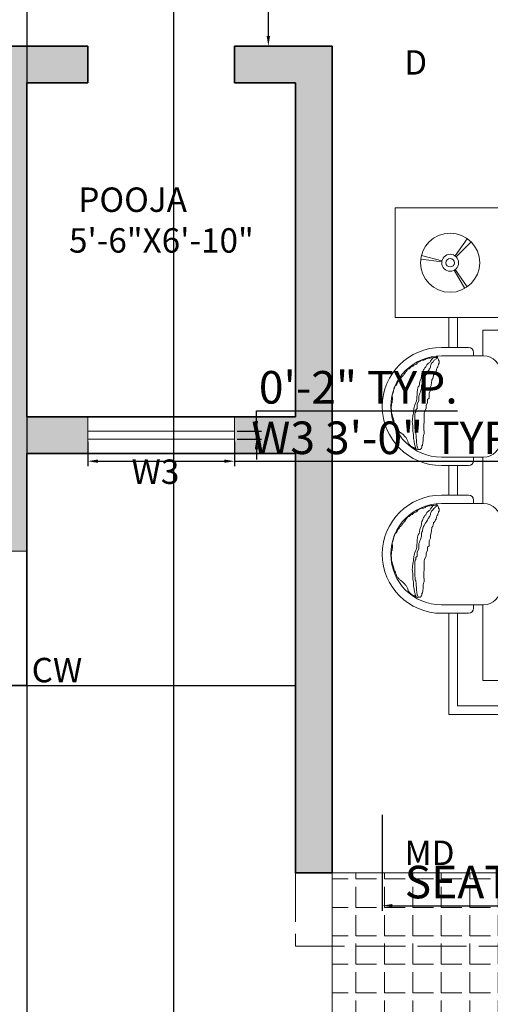
# Model space of a CAD drawing. Units: inches. Extents: x 1070 to 2371, y 645 to 1546.
# Tile 3 of 10: x 1342 to 1458, y 772 to 1014. Entities that reach past the tile are written whole.
import ezdxf

# ---------------------------------------------------------------- set-up
doc = ezdxf.new("R2010")
doc.units = ezdxf.units.IN
doc.linetypes.add('ACAD_ISO02W100', pattern=[15, 12, -3])
for name, color, linetype, lineweight in [('A-ANNO-DIMS', 2, 'Continuous', 18), ('A-ANNO-TEXT', 7, 'Continuous', 18), ('A-AREA-IDEN', 7, 'Continuous', 18), ('A-DOOR', 4, 'Continuous', 18), ('A-FLOR', 7, 'Continuous', 25), ('A-FURN', 8, 'Continuous', 18), ('A-GLAZ', 4, 'Continuous', 18), ('A-ROOF-OVHD', 8, 'ACAD_ISO02W100', 13), ('A-WALL', 7, 'Continuous', 35), ('L-PLNT-BEDS', 3, 'Continuous', 18), ('L-TURF-PATT', 9, 'Continuous', 13)]:
    doc.layers.add(name, color=color, linetype=linetype, lineweight=lineweight)
doc.layers.add('A-WALL-PATT', color=162, linetype='Continuous', lineweight=13, true_color=0x044ac3)
doc.styles.get("Standard").update_dxf_attribs({"font": 'arial.ttf'})
doc.dimstyles.new('ISO-25', dxfattribs={"dimtxt": 8, "dimasz": 2.5, "dimexe": 1.25, "dimexo": 0.625, "dimtad": 1, "dimtih": 1, "dimtoh": 1, "dimdec": 1, "dimlunit": 3, "dimtxsty": 'Standard', "dimcen": 2.5, "dimadec": 0, "dimazin": 0, "dimtfac": 1, "dimtdec": 1, "dimtmove": 0, "dimatfit": 3, "dimfxl": 1, "dimarcsym": 0})

# ---------------------------------------------------------------- blocks, each defined once
blk = doc.blocks.new('A$C71DE5BFE')
for p, q in [((430.7, 3295.7), (503.4, 3397.4)), ((437, 3290.4), (525.4, 3378.7)), ((352, 3261.2), (228, 3276.7)), ((353.2, 3267.1), (231.9, 3297.4)), ((426.5, 3211.6), (488.5, 3103.1)), ((430.7, 3214.3), (503.4, 3112.6)), ((394.4, 2753.9), (394.4, 2930)), ((444.4, 2753.9), (444.4, 2930)), ((350, 2753.9), (510, 2753.9)), ((254.6, 2681.5), (256.9, 2686.1)), ((256.9, 2686.1), (261.2, 2686.1)), ((261.2, 2686.1), (265.5, 2688.1)), ((265.5, 2688.1), (270.1, 2688.1)), ((270.1, 2688.1), (274.4, 2690.5)), ((274.4, 2690.5), (283.1, 2690.5)), ((283.1, 2690.5), (287.7, 2692.5)), ((287.7, 2692.5), (305, 2692.5)), ((292, 2681.5), (296.3, 2686.1)), ((296.3, 2686.1), (298.6, 2690.5)), ((298.6, 2690.5), (300.7, 2694.8)), ((300.7, 2694.8), (303, 2694.8)), ((305, 2692.5), (309.6, 2694.8)), ((309.6, 2694.8), (322.6, 2694.8)), ((315.9, 2683.8), (311.6, 2681.5)), ((320.5, 2686.1), (315.9, 2683.8)), ((318.2, 2697.1), (322.6, 2697.1)), ((322.6, 2690.5), (320.5, 2686.1)), ((322.6, 2694.8), (326.9, 2697.1)), ((322.6, 2697.1), (326.9, 2694.8)), ((326.9, 2694.8), (322.6, 2690.5)), ((326.9, 2697.1), (329.2, 2697.1)), ((326.9, 2694.8), (331.5, 2686.1)), ((331.5, 2686.1), (333.5, 2681.5)), ((350, 2703.9), (600, 2703.9)), ((540, 2723.9), (540, 2703.9)), ((149.4, 2622.4), (154, 2624.7)), ((154, 2624.7), (158.3, 2626.7)), ((158.3, 2626.7), (162.6, 2631.3)), ((162.6, 2631.3), (166.9, 2635.6)), ((166.9, 2635.6), (171.3, 2637.7)), ((171.3, 2637.7), (175.9, 2640)), ((175.9, 2640), (180.2, 2642.3)), ((180.2, 2642.3), (184.5, 2646.6)), ((184.5, 2646.6), (188.8, 2648.6)), ((188.8, 2648.6), (193.5, 2650.9)), ((193.5, 2650.9), (197.8, 2653.2)), ((197.8, 2653.2), (202.1, 2655.3)), ((202.1, 2655.3), (206.4, 2659.6)), ((206.4, 2659.6), (210.7, 2661.9)), ((210.7, 2661.9), (213.1, 2666.2)), ((213.1, 2666.2), (217.4, 2668.5)), ((217.4, 2668.5), (219.7, 2672.9)), ((219.7, 2672.9), (224, 2672.9)), ((224, 2672.9), (228.3, 2675.2)), ((228.3, 2675.2), (232.7, 2677.2)), ((232.7, 2677.2), (245.9, 2677.2)), ((243.6, 2620.4), (248.2, 2624.7)), ((245.9, 2677.2), (250.2, 2679.5)), ((248.2, 2624.7), (250.2, 2629)), ((250.2, 2679.5), (254.6, 2681.5)), ((250.2, 2629), (252.5, 2633.3)), ((252.5, 2633.3), (256.9, 2637.7)), ((256.9, 2637.7), (259.2, 2642.3)), ((259.2, 2642.3), (261.2, 2646.6)), ((261.2, 2646.6), (263.5, 2650.9)), ((263.5, 2650.9), (267.8, 2655.3)), ((267.8, 2655.3), (272.1, 2657.6)), ((272.1, 2657.6), (276.5, 2661.9)), ((276.5, 2661.9), (281.1, 2664.2)), ((281.1, 2629), (276.5, 2624.7)), ((276.5, 2624.7), (276.5, 2620.4)), ((281.1, 2664.2), (283.1, 2668.5)), ((283.1, 2633.3), (281.1, 2629)), ((283.1, 2668.5), (285.4, 2672.9)), ((285.4, 2637.7), (283.1, 2633.3)), ((285.4, 2672.9), (289.7, 2677.2)), ((287.7, 2648.6), (285.4, 2644.3)), ((285.4, 2644.3), (285.4, 2637.7)), ((289.7, 2655.3), (287.7, 2648.6)), ((289.7, 2677.2), (292, 2681.5)), ((292, 2659.6), (289.7, 2655.3)), ((296.3, 2664.2), (292, 2659.6)), ((300.7, 2668.5), (296.3, 2664.2)), ((305, 2675.2), (300.7, 2668.5)), ((309.6, 2677.2), (305, 2675.2)), ((311.6, 2681.5), (309.6, 2677.2)), ((322.6, 2629), (320.5, 2624.7)), ((320.5, 2624.7), (320.5, 2620.4)), ((324.9, 2633.3), (322.6, 2629)), ((329.2, 2637.7), (324.9, 2633.3)), ((331.5, 2646.6), (329.2, 2642.3)), ((329.2, 2642.3), (329.2, 2637.7)), ((333.5, 2650.9), (331.5, 2646.6)), ((333.5, 2681.5), (333.5, 2677.2)), ((333.5, 2677.2), (335.8, 2672.9)), ((335.8, 2659.6), (333.5, 2655.3)), ((333.5, 2655.3), (333.5, 2650.9)), ((335.8, 2672.9), (335.8, 2659.6)), ((103.5, 2563.2), (105.6, 2567.6)), ((105.6, 2567.6), (110.2, 2567.6)), ((110.2, 2572.2), (114.5, 2574.2)), ((110.2, 2567.6), (110.2, 2572.2)), ((114.5, 2574.2), (116.5, 2578.5)), ((116.5, 2578.5), (118.8, 2583.1)), ((118.8, 2583.1), (123.1, 2585.2)), ((123.1, 2589.5), (127.5, 2591.8)), ((123.1, 2585.2), (123.1, 2589.5)), ((127.5, 2591.8), (129.8, 2596.1)), ((129.8, 2596.1), (134.1, 2600.5)), ((134.1, 2600.5), (136.4, 2605.1)), ((136.4, 2605.1), (138.4, 2609.4)), ((138.4, 2609.4), (143, 2611.4)), ((143, 2615.7), (147.3, 2618)), ((143, 2611.4), (143, 2615.7)), ((147.3, 2618), (149.4, 2622.4)), ((228.3, 2565.5), (230.6, 2569.9)), ((230.6, 2574.2), (232.7, 2580.8)), ((230.6, 2569.9), (230.6, 2574.2)), ((232.7, 2589.5), (235, 2594.1)), ((232.7, 2580.8), (232.7, 2589.5)), ((235, 2598.4), (237.3, 2602.8)), ((235, 2594.1), (235, 2598.4)), ((237.3, 2602.8), (239.3, 2607.1)), ((239.3, 2611.4), (241.6, 2615.7)), ((239.3, 2607.1), (239.3, 2611.4)), ((241.6, 2615.7), (243.6, 2620.4)), ((243.6, 2567.6), (241.6, 2561.2)), ((248.2, 2574.2), (243.6, 2567.6)), ((250.2, 2578.5), (248.2, 2574.2)), ((254.6, 2585.2), (250.2, 2578.5)), ((259.2, 2594.1), (254.6, 2585.2)), ((267.8, 2605.1), (259.2, 2594.1)), ((272.1, 2615.7), (267.8, 2605.1)), ((276.5, 2620.4), (272.1, 2615.7)), ((298.6, 2569.9), (294, 2561.2)), ((300.7, 2578.5), (298.6, 2569.9)), ((303, 2585.2), (300.7, 2578.5)), ((311.6, 2598.4), (303, 2589.5)), ((303, 2589.5), (303, 2585.2)), ((315.9, 2607.1), (311.6, 2598.4)), ((318.2, 2611.4), (315.9, 2607.1)), ((320.5, 2620.4), (318.2, 2615.7)), ((318.2, 2615.7), (318.2, 2611.4)), ((68.4, 2510.7), (70.7, 2515.1)), ((68.4, 2502.1), (68.4, 2510.7)), ((70.7, 2515.1), (72.7, 2519.4)), ((72.7, 2519.4), (75, 2523.7)), ((75, 2523.7), (79.3, 2528.3)), ((79.3, 2528.3), (83.7, 2530.4)), ((83.7, 2530.4), (86, 2534.7)), ((86, 2534.7), (88.3, 2539.3)), ((88.3, 2539.3), (90.3, 2543.6)), ((90.3, 2543.6), (92.6, 2547.9)), ((92.6, 2547.9), (94.6, 2552.3)), ((94.6, 2552.3), (99.2, 2556.6)), ((99.2, 2561.2), (103.5, 2563.2)), ((99.2, 2556.6), (99.2, 2561.2)), ((208.7, 2506.4), (210.7, 2510.7)), ((210.7, 2515.1), (213.1, 2519.4)), ((210.7, 2510.7), (210.7, 2515.1)), ((213.1, 2519.4), (217.4, 2526)), ((217.4, 2530.4), (219.7, 2534.7)), ((217.4, 2526), (217.4, 2530.4)), ((219.7, 2541.3), (221.7, 2547.9)), ((219.7, 2534.7), (219.7, 2541.3)), ((221.7, 2552.3), (224, 2556.6)), ((221.7, 2547.9), (221.7, 2552.3)), ((224, 2556.6), (226.3, 2561.2)), ((226.3, 2561.2), (228.3, 2565.5)), ((232.7, 2510.7), (230.6, 2504.1)), ((235, 2534.7), (232.7, 2530.4)), ((232.7, 2530.4), (232.7, 2510.7)), ((237.3, 2541.3), (235, 2534.7)), ((239.3, 2552.3), (237.3, 2545.6)), ((237.3, 2545.6), (237.3, 2541.3)), ((241.6, 2561.2), (239.3, 2556.6)), ((239.3, 2556.6), (239.3, 2552.3)), ((289.7, 2528.3), (285.4, 2519.4)), ((285.4, 2519.4), (285.4, 2499.8)), ((292, 2541.3), (289.7, 2534.7)), ((289.7, 2534.7), (289.7, 2528.3)), ((294, 2556.6), (292, 2547.9)), ((292, 2547.9), (292, 2541.3)), ((294, 2561.2), (294, 2556.6)), ((57.4, 2471.2), (59.7, 2475.5)), ((57.4, 2462.6), (57.4, 2471.2)), ((59.7, 2458.2), (57.4, 2462.6)), ((59.7, 2475.5), (61.8, 2480.2)), ((59.7, 2440.6), (59.7, 2458.2)), ((61.8, 2480.2), (64.1, 2484.5)), ((64.1, 2488.8), (66.4, 2493.1)), ((64.1, 2484.5), (64.1, 2488.8)), ((66.4, 2497.5), (68.4, 2502.1)), ((66.4, 2493.1), (66.4, 2497.5)), ((204.4, 2464.6), (206.4, 2469.2)), ((204.4, 2445), (204.4, 2464.6)), ((206.4, 2493.1), (208.7, 2497.5)), ((206.4, 2469.2), (206.4, 2493.1)), ((208.7, 2497.5), (208.7, 2506.4)), ((217.4, 2471.2), (215.4, 2466.9)), ((215.4, 2466.9), (215.4, 2436.3)), ((219.7, 2475.5), (217.4, 2471.2)), ((221.7, 2482.2), (219.7, 2475.5)), ((224, 2486.5), (221.7, 2482.2)), ((226.3, 2491.1), (224, 2486.5)), ((228.3, 2497.5), (226.3, 2491.1)), ((230.6, 2504.1), (228.3, 2497.5)), ((276.5, 2453.6), (267.8, 2445)), ((285.4, 2499.8), (276.5, 2482.2)), ((276.5, 2482.2), (276.5, 2453.6)), ((53.1, 2401.1), (55.1, 2405.4)), ((53.1, 2392.5), (53.1, 2401.1)), ((55.1, 2388.1), (53.1, 2392.5)), ((55.1, 2423), (57.4, 2427.4)), ((55.1, 2405.4), (55.1, 2423)), ((57.4, 2436.3), (59.7, 2440.6)), ((57.4, 2427.4), (57.4, 2436.3)), ((186.8, 2392.5), (188.8, 2396.8)), ((186.8, 2381.5), (186.8, 2392.5)), ((188.8, 2401.1), (191.2, 2405.4)), ((188.8, 2396.8), (188.8, 2401.1)), ((191.2, 2405.4), (193.5, 2414.4)), ((193.5, 2414.4), (197.8, 2427.4)), ((197.8, 2427.4), (199.8, 2431.7)), ((206.4, 2392.5), (197.8, 2383.5)), ((199.8, 2431.7), (202.1, 2436.3)), ((202.1, 2440.6), (204.4, 2445)), ((202.1, 2436.3), (202.1, 2440.6)), ((215.4, 2436.3), (206.4, 2418.7)), ((206.4, 2418.7), (206.4, 2392.5)), ((259.2, 2392.5), (250.2, 2374.9)), ((267.8, 2427.4), (259.2, 2410.1)), ((259.2, 2410.1), (259.2, 2392.5)), ((267.8, 2445), (267.8, 2427.4)), ((55.1, 2361.6), (55.1, 2388.1)), ((57.4, 2357.3), (55.1, 2361.6)), ((57.4, 2352.9), (57.4, 2357.3)), ((59.7, 2348.6), (57.4, 2352.9)), ((59.7, 2344.3), (59.7, 2348.6)), ((61.8, 2340), (59.7, 2344.3)), ((64.1, 2335.3), (61.8, 2340)), ((66.4, 2331), (64.1, 2335.3)), ((177.9, 2335.3), (180.2, 2342)), ((177.9, 2322.4), (177.9, 2335.3)), ((180.2, 2350.6), (182.5, 2357.3)), ((180.2, 2342), (180.2, 2350.6)), ((182.5, 2357.3), (184.5, 2363.9)), ((184.5, 2377.2), (186.8, 2381.5)), ((184.5, 2363.9), (184.5, 2377.2)), ((195.5, 2363.9), (193.5, 2359.6)), ((193.5, 2359.6), (193.5, 2274.2)), ((197.8, 2372.6), (195.5, 2368.2)), ((195.5, 2368.2), (195.5, 2363.9)), ((197.8, 2383.5), (197.8, 2372.6)), ((250.2, 2370.5), (248.2, 2366.2)), ((248.2, 2366.2), (248.2, 2307.1)), ((250.2, 2374.9), (250.2, 2370.5)), ((66.4, 2326.7), (66.4, 2331)), ((68.4, 2322.4), (66.4, 2326.7)), ((68.4, 2318), (68.4, 2322.4)), ((70.7, 2311.4), (68.4, 2318)), ((72.7, 2307.1), (70.7, 2311.4)), ((75, 2302.5), (72.7, 2307.1)), ((77.3, 2298.1), (75, 2302.5)), ((77.3, 2293.8), (77.3, 2298.1)), ((79.3, 2289.5), (77.3, 2293.8)), ((81.6, 2285.1), (79.3, 2289.5)), ((83.7, 2278.5), (81.6, 2285.1)), ((86, 2274.2), (83.7, 2278.5)), ((175.9, 2315.7), (177.9, 2322.4)), ((175.9, 2311.4), (175.9, 2315.7)), ((177.9, 2307.1), (175.9, 2311.4)), ((177.9, 2298.1), (177.9, 2307.1)), ((180.2, 2293.8), (177.9, 2298.1)), ((180.2, 2254.3), (180.2, 2293.8)), ((248.2, 2307.1), (245.9, 2300.4)), ((245.9, 2300.4), (245.9, 2263.2)), ((88.3, 2269.6), (86, 2274.2)), ((90.3, 2265.2), (88.3, 2269.6)), ((94.6, 2263.2), (90.3, 2265.2)), ((96.9, 2258.6), (94.6, 2263.2)), ((101.2, 2256.6), (96.9, 2258.6)), ((103.5, 2252.3), (101.2, 2256.6)), ((107.9, 2250), (103.5, 2252.3)), ((112.2, 2245.6), (107.9, 2250)), ((121.1, 2239), (112.2, 2245.6)), ((134.1, 2226), (121.1, 2239)), ((136.4, 2221.4), (134.1, 2226)), ((140.7, 2219.4), (136.4, 2221.4)), ((143, 2215), (140.7, 2219.4)), ((182.5, 2250), (180.2, 2254.3)), ((182.5, 2245.6), (182.5, 2250)), ((184.5, 2239), (182.5, 2245.6)), ((184.5, 2212.7), (184.5, 2239)), ((193.5, 2274.2), (195.5, 2265.2)), ((195.5, 2265.2), (195.5, 2252.3)), ((195.5, 2252.3), (197.8, 2247.9)), ((197.8, 2247.9), (197.8, 2243.3)), ((197.8, 2243.3), (199.8, 2232.4)), ((199.8, 2232.4), (199.8, 2215)), ((243.6, 2228), (241.6, 2223.7)), ((241.6, 2223.7), (241.6, 2197.5)), ((245.9, 2237), (243.6, 2232.4)), ((243.6, 2232.4), (243.6, 2228)), ((245.9, 2263.2), (248.2, 2258.6)), ((248.2, 2241.3), (245.9, 2237)), ((248.2, 2258.6), (248.2, 2241.3)), ((145, 2210.4), (143, 2215)), ((147.3, 2206.1), (145, 2210.4)), ((149.4, 2201.8), (147.3, 2206.1)), ((151.7, 2197.5), (149.4, 2201.8)), ((154, 2190.8), (151.7, 2197.5)), ((154, 2186.5), (154, 2190.8)), ((156, 2182.2), (154, 2186.5)), ((160.3, 2179.9), (156, 2182.2)), ((162.6, 2175.5), (160.3, 2179.9)), ((166.9, 2171.2), (162.6, 2175.5)), ((169.2, 2166.6), (166.9, 2171.2)), ((173.6, 2166.6), (169.2, 2166.6)), ((175.9, 2162.3), (173.6, 2166.6)), ((180.2, 2162.3), (175.9, 2162.3)), ((184.5, 2160.2), (180.2, 2162.3)), ((186.8, 2208.4), (184.5, 2212.7)), ((188.8, 2157.9), (184.5, 2160.2)), ((186.8, 2204.1), (186.8, 2208.4)), ((188.8, 2199.5), (186.8, 2204.1)), ((188.8, 2190.8), (188.8, 2199.5)), ((191.2, 2186.5), (188.8, 2190.8)), ((195.5, 2153.6), (188.8, 2157.9)), ((191.2, 2179.9), (191.2, 2186.5)), ((193.5, 2175.5), (191.2, 2179.9)), ((195.5, 2171.2), (193.5, 2175.5)), ((195.5, 2162.3), (195.5, 2171.2)), ((197.8, 2157.9), (195.5, 2162.3)), ((199.8, 2153.6), (197.8, 2157.9)), ((199.8, 2215), (202.1, 2208.4)), ((202.1, 2208.4), (202.1, 2186.5)), ((202.1, 2186.5), (204.4, 2182.2)), ((204.4, 2182.2), (204.4, 2173.2)), ((204.4, 2173.2), (206.4, 2168.9)), ((206.4, 2168.9), (206.4, 2164.6)), ((206.4, 2164.6), (208.7, 2160.2)), ((208.7, 2160.2), (210.7, 2155.9)), ((232.7, 2157.9), (228.3, 2153.6)), ((235, 2162.3), (232.7, 2157.9)), ((237.3, 2175.5), (235, 2171.2)), ((235, 2171.2), (235, 2162.3)), ((239.3, 2184.2), (237.3, 2179.9)), ((237.3, 2179.9), (237.3, 2175.5)), ((241.6, 2197.5), (239.3, 2193.1)), ((239.3, 2193.1), (239.3, 2184.2)), ((199.8, 2151.3), (195.5, 2153.6)), ((199.8, 2149.3), (199.8, 2153.6)), ((204.4, 2149.3), (199.8, 2151.3)), ((208.7, 2147), (204.4, 2149.3)), ((213.1, 2149.3), (208.7, 2147)), ((210.7, 2155.9), (213.1, 2151.3)), ((213.1, 2151.3), (213.1, 2149.3)), ((226.3, 2149.3), (213.1, 2149.3)), ((228.3, 2153.6), (226.3, 2149.3)), ((350, 2103.9), (600, 2103.9)), ((540, 2103.9), (540, 2083.9)), ((594.4, 1828.9), (594.4, 2103.9)), ((510, 2053.9), (350, 2053.9)), ((394.4, 1878.9), (394.4, 2053.9)), ((444.4, 1878.9), (444.4, 2053.9)), ((350, 1878.9), (510, 1878.9)), ((254.6, 1806.5), (256.9, 1811.1)), ((256.9, 1811.1), (261.2, 1811.1)), ((261.2, 1811.1), (265.5, 1813.1)), ((265.5, 1813.1), (270.1, 1813.1)), ((270.1, 1813.1), (274.4, 1815.5)), ((274.4, 1815.5), (283.1, 1815.5)), ((283.1, 1815.5), (287.7, 1817.5)), ((287.7, 1817.5), (305, 1817.5)), ((292, 1806.5), (296.3, 1811.1)), ((296.3, 1811.1), (298.6, 1815.5)), ((298.6, 1815.5), (300.7, 1819.8)), ((300.7, 1819.8), (303, 1819.8)), ((305, 1817.5), (309.6, 1819.8)), ((309.6, 1819.8), (322.6, 1819.8)), ((315.9, 1808.8), (311.6, 1806.5)), ((320.5, 1811.1), (315.9, 1808.8)), ((318.2, 1822.1), (322.6, 1822.1)), ((322.6, 1815.5), (320.5, 1811.1)), ((322.6, 1819.8), (326.9, 1822.1)), ((322.6, 1822.1), (326.9, 1819.8)), ((326.9, 1819.8), (322.6, 1815.5)), ((326.9, 1822.1), (329.2, 1822.1)), ((326.9, 1819.8), (331.5, 1811.1)), ((331.5, 1811.1), (333.5, 1806.5)), ((350, 1828.9), (600, 1828.9)), ((540, 1848.9), (540, 1828.9)), ((149.4, 1747.4), (154, 1749.7)), ((154, 1749.7), (158.3, 1751.7)), ((158.3, 1751.7), (162.6, 1756.3)), ((162.6, 1756.3), (166.9, 1760.6)), ((166.9, 1760.6), (171.3, 1762.7)), ((171.3, 1762.7), (175.9, 1765)), ((175.9, 1765), (180.2, 1767.3)), ((180.2, 1767.3), (184.5, 1771.6)), ((184.5, 1771.6), (188.8, 1773.6)), ((188.8, 1773.6), (193.5, 1775.9)), ((193.5, 1775.9), (197.8, 1778.2)), ((197.8, 1778.2), (202.1, 1780.3)), ((202.1, 1780.3), (206.4, 1784.6)), ((206.4, 1784.6), (210.7, 1786.9)), ((210.7, 1786.9), (213.1, 1791.2)), ((213.1, 1791.2), (217.4, 1793.5)), ((217.4, 1793.5), (219.7, 1797.9)), ((219.7, 1797.9), (224, 1797.9)), ((224, 1797.9), (228.3, 1800.2)), ((228.3, 1800.2), (232.7, 1802.2)), ((232.7, 1802.2), (245.9, 1802.2)), ((243.6, 1745.4), (248.2, 1749.7)), ((245.9, 1802.2), (250.2, 1804.5)), ((248.2, 1749.7), (250.2, 1754)), ((250.2, 1804.5), (254.6, 1806.5)), ((250.2, 1754), (252.5, 1758.3)), ((252.5, 1758.3), (256.9, 1762.7)), ((256.9, 1762.7), (259.2, 1767.3)), ((259.2, 1767.3), (261.2, 1771.6)), ((261.2, 1771.6), (263.5, 1775.9)), ((263.5, 1775.9), (267.8, 1780.3)), ((267.8, 1780.3), (272.1, 1782.6)), ((272.1, 1782.6), (276.5, 1786.9)), ((276.5, 1786.9), (281.1, 1789.2)), ((281.1, 1754), (276.5, 1749.7)), ((276.5, 1749.7), (276.5, 1745.4)), ((281.1, 1789.2), (283.1, 1793.5)), ((283.1, 1758.3), (281.1, 1754)), ((283.1, 1793.5), (285.4, 1797.9)), ((285.4, 1762.7), (283.1, 1758.3)), ((285.4, 1797.9), (289.7, 1802.2)), ((287.7, 1773.6), (285.4, 1769.3)), ((285.4, 1769.3), (285.4, 1762.7)), ((289.7, 1780.3), (287.7, 1773.6)), ((289.7, 1802.2), (292, 1806.5)), ((292, 1784.6), (289.7, 1780.3)), ((296.3, 1789.2), (292, 1784.6)), ((300.7, 1793.5), (296.3, 1789.2)), ((305, 1800.2), (300.7, 1793.5)), ((309.6, 1802.2), (305, 1800.2)), ((311.6, 1806.5), (309.6, 1802.2)), ((322.6, 1754), (320.5, 1749.7)), ((320.5, 1749.7), (320.5, 1745.4)), ((324.9, 1758.3), (322.6, 1754)), ((329.2, 1762.7), (324.9, 1758.3)), ((331.5, 1771.6), (329.2, 1767.3)), ((329.2, 1767.3), (329.2, 1762.7)), ((333.5, 1775.9), (331.5, 1771.6)), ((333.5, 1806.5), (333.5, 1802.2)), ((333.5, 1802.2), (335.8, 1797.9)), ((335.8, 1784.6), (333.5, 1780.3)), ((333.5, 1780.3), (333.5, 1775.9)), ((335.8, 1797.9), (335.8, 1784.6)), ((103.5, 1688.2), (105.6, 1692.6)), ((105.6, 1692.6), (110.2, 1692.6)), ((110.2, 1697.2), (114.5, 1699.2)), ((110.2, 1692.6), (110.2, 1697.2)), ((114.5, 1699.2), (116.5, 1703.5)), ((116.5, 1703.5), (118.8, 1708.1)), ((118.8, 1708.1), (123.1, 1710.2)), ((123.1, 1714.5), (127.5, 1716.8)), ((123.1, 1710.2), (123.1, 1714.5)), ((127.5, 1716.8), (129.8, 1721.1)), ((129.8, 1721.1), (134.1, 1725.5)), ((134.1, 1725.5), (136.4, 1730.1)), ((136.4, 1730.1), (138.4, 1734.4)), ((138.4, 1734.4), (143, 1736.4)), ((143, 1740.7), (147.3, 1743)), ((143, 1736.4), (143, 1740.7)), ((147.3, 1743), (149.4, 1747.4)), ((228.3, 1690.5), (230.6, 1694.9)), ((230.6, 1699.2), (232.7, 1705.8)), ((230.6, 1694.9), (230.6, 1699.2)), ((232.7, 1714.5), (235, 1719.1)), ((232.7, 1705.8), (232.7, 1714.5)), ((235, 1723.4), (237.3, 1727.8)), ((235, 1719.1), (235, 1723.4)), ((237.3, 1727.8), (239.3, 1732.1)), ((239.3, 1736.4), (241.6, 1740.7)), ((239.3, 1732.1), (239.3, 1736.4)), ((241.6, 1740.7), (243.6, 1745.4)), ((243.6, 1692.6), (241.6, 1686.2)), ((248.2, 1699.2), (243.6, 1692.6)), ((250.2, 1703.5), (248.2, 1699.2)), ((254.6, 1710.2), (250.2, 1703.5)), ((259.2, 1719.1), (254.6, 1710.2)), ((267.8, 1730.1), (259.2, 1719.1)), ((272.1, 1740.7), (267.8, 1730.1)), ((276.5, 1745.4), (272.1, 1740.7)), ((298.6, 1694.9), (294, 1686.2)), ((300.7, 1703.5), (298.6, 1694.9)), ((303, 1710.2), (300.7, 1703.5)), ((311.6, 1723.4), (303, 1714.5)), ((303, 1714.5), (303, 1710.2)), ((315.9, 1732.1), (311.6, 1723.4)), ((318.2, 1736.4), (315.9, 1732.1)), ((320.5, 1745.4), (318.2, 1740.7)), ((318.2, 1740.7), (318.2, 1736.4)), ((68.4, 1635.7), (70.7, 1640.1)), ((68.4, 1627.1), (68.4, 1635.7)), ((70.7, 1640.1), (72.7, 1644.4)), ((72.7, 1644.4), (75, 1648.7)), ((75, 1648.7), (79.3, 1653.3)), ((79.3, 1653.3), (83.7, 1655.4)), ((83.7, 1655.4), (86, 1659.7)), ((86, 1659.7), (88.3, 1664.3)), ((88.3, 1664.3), (90.3, 1668.6)), ((90.3, 1668.6), (92.6, 1672.9)), ((92.6, 1672.9), (94.6, 1677.3)), ((94.6, 1677.3), (99.2, 1681.6)), ((99.2, 1686.2), (103.5, 1688.2)), ((99.2, 1681.6), (99.2, 1686.2)), ((208.7, 1631.4), (210.7, 1635.7)), ((210.7, 1640.1), (213.1, 1644.4)), ((210.7, 1635.7), (210.7, 1640.1)), ((213.1, 1644.4), (217.4, 1651)), ((217.4, 1655.4), (219.7, 1659.7)), ((217.4, 1651), (217.4, 1655.4)), ((219.7, 1666.3), (221.7, 1672.9)), ((219.7, 1659.7), (219.7, 1666.3)), ((221.7, 1677.3), (224, 1681.6)), ((221.7, 1672.9), (221.7, 1677.3)), ((224, 1681.6), (226.3, 1686.2)), ((226.3, 1686.2), (228.3, 1690.5)), ((232.7, 1635.7), (230.6, 1629.1)), ((235, 1659.7), (232.7, 1655.4)), ((232.7, 1655.4), (232.7, 1635.7)), ((237.3, 1666.3), (235, 1659.7)), ((239.3, 1677.3), (237.3, 1670.6)), ((237.3, 1670.6), (237.3, 1666.3)), ((241.6, 1686.2), (239.3, 1681.6)), ((239.3, 1681.6), (239.3, 1677.3)), ((289.7, 1653.3), (285.4, 1644.4)), ((285.4, 1644.4), (285.4, 1624.8)), ((292, 1666.3), (289.7, 1659.7)), ((289.7, 1659.7), (289.7, 1653.3)), ((294, 1681.6), (292, 1672.9)), ((292, 1672.9), (292, 1666.3)), ((294, 1686.2), (294, 1681.6)), ((57.4, 1596.2), (59.7, 1600.5)), ((57.4, 1587.6), (57.4, 1596.2)), ((59.7, 1583.2), (57.4, 1587.6)), ((59.7, 1600.5), (61.8, 1605.2)), ((59.7, 1565.6), (59.7, 1583.2)), ((61.8, 1605.2), (64.1, 1609.5)), ((64.1, 1613.8), (66.4, 1618.1)), ((64.1, 1609.5), (64.1, 1613.8)), ((66.4, 1622.5), (68.4, 1627.1)), ((66.4, 1618.1), (66.4, 1622.5)), ((204.4, 1589.6), (206.4, 1594.2)), ((204.4, 1570), (204.4, 1589.6)), ((206.4, 1618.1), (208.7, 1622.5)), ((206.4, 1594.2), (206.4, 1618.1)), ((208.7, 1622.5), (208.7, 1631.4)), ((217.4, 1596.2), (215.4, 1591.9)), ((215.4, 1591.9), (215.4, 1561.3)), ((219.7, 1600.5), (217.4, 1596.2)), ((221.7, 1607.2), (219.7, 1600.5)), ((224, 1611.5), (221.7, 1607.2)), ((226.3, 1616.1), (224, 1611.5)), ((228.3, 1622.5), (226.3, 1616.1)), ((230.6, 1629.1), (228.3, 1622.5)), ((276.5, 1578.6), (267.8, 1570)), ((285.4, 1624.8), (276.5, 1607.2)), ((276.5, 1607.2), (276.5, 1578.6)), ((53.1, 1526.1), (55.1, 1530.4)), ((53.1, 1517.5), (53.1, 1526.1)), ((55.1, 1513.1), (53.1, 1517.5)), ((55.1, 1548), (57.4, 1552.4)), ((55.1, 1530.4), (55.1, 1548)), ((57.4, 1561.3), (59.7, 1565.6)), ((57.4, 1552.4), (57.4, 1561.3)), ((186.8, 1517.5), (188.8, 1521.8)), ((186.8, 1506.5), (186.8, 1517.5)), ((188.8, 1526.1), (191.2, 1530.4)), ((188.8, 1521.8), (188.8, 1526.1)), ((191.2, 1530.4), (193.5, 1539.4)), ((193.5, 1539.4), (197.8, 1552.4)), ((197.8, 1552.4), (199.8, 1556.7)), ((206.4, 1517.5), (197.8, 1508.5)), ((199.8, 1556.7), (202.1, 1561.3)), ((202.1, 1565.6), (204.4, 1570)), ((202.1, 1561.3), (202.1, 1565.6)), ((215.4, 1561.3), (206.4, 1543.7)), ((206.4, 1543.7), (206.4, 1517.5)), ((259.2, 1517.5), (250.2, 1499.9)), ((267.8, 1552.4), (259.2, 1535.1)), ((259.2, 1535.1), (259.2, 1517.5)), ((267.8, 1570), (267.8, 1552.4)), ((55.1, 1486.6), (55.1, 1513.1)), ((57.4, 1482.3), (55.1, 1486.6)), ((57.4, 1477.9), (57.4, 1482.3)), ((59.7, 1473.6), (57.4, 1477.9)), ((59.7, 1469.3), (59.7, 1473.6)), ((61.8, 1465), (59.7, 1469.3)), ((64.1, 1460.3), (61.8, 1465)), ((66.4, 1456), (64.1, 1460.3)), ((177.9, 1460.3), (180.2, 1467)), ((177.9, 1447.4), (177.9, 1460.3)), ((180.2, 1475.6), (182.5, 1482.3)), ((180.2, 1467), (180.2, 1475.6)), ((182.5, 1482.3), (184.5, 1488.9)), ((184.5, 1502.2), (186.8, 1506.5)), ((184.5, 1488.9), (184.5, 1502.2)), ((195.5, 1488.9), (193.5, 1484.6)), ((193.5, 1484.6), (193.5, 1399.2)), ((197.8, 1497.6), (195.5, 1493.2)), ((195.5, 1493.2), (195.5, 1488.9)), ((197.8, 1508.5), (197.8, 1497.6)), ((250.2, 1495.5), (248.2, 1491.2)), ((248.2, 1491.2), (248.2, 1432.1)), ((250.2, 1499.9), (250.2, 1495.5)), ((66.4, 1451.7), (66.4, 1456)), ((68.4, 1447.4), (66.4, 1451.7)), ((68.4, 1443), (68.4, 1447.4)), ((70.7, 1436.4), (68.4, 1443)), ((72.7, 1432.1), (70.7, 1436.4)), ((75, 1427.5), (72.7, 1432.1)), ((77.3, 1423.1), (75, 1427.5)), ((77.3, 1418.8), (77.3, 1423.1)), ((79.3, 1414.5), (77.3, 1418.8)), ((81.6, 1410.1), (79.3, 1414.5)), ((83.7, 1403.5), (81.6, 1410.1)), ((86, 1399.2), (83.7, 1403.5)), ((175.9, 1440.7), (177.9, 1447.4)), ((175.9, 1436.4), (175.9, 1440.7)), ((177.9, 1432.1), (175.9, 1436.4)), ((177.9, 1423.1), (177.9, 1432.1)), ((180.2, 1418.8), (177.9, 1423.1)), ((180.2, 1379.3), (180.2, 1418.8)), ((248.2, 1432.1), (245.9, 1425.4)), ((245.9, 1425.4), (245.9, 1388.2)), ((88.3, 1394.6), (86, 1399.2)), ((90.3, 1390.2), (88.3, 1394.6)), ((94.6, 1388.2), (90.3, 1390.2)), ((96.9, 1383.6), (94.6, 1388.2)), ((101.2, 1381.6), (96.9, 1383.6)), ((103.5, 1377.3), (101.2, 1381.6)), ((107.9, 1375), (103.5, 1377.3)), ((112.2, 1370.6), (107.9, 1375)), ((121.1, 1364), (112.2, 1370.6)), ((134.1, 1351), (121.1, 1364)), ((136.4, 1346.4), (134.1, 1351)), ((140.7, 1344.4), (136.4, 1346.4)), ((143, 1340), (140.7, 1344.4)), ((182.5, 1375), (180.2, 1379.3)), ((182.5, 1370.6), (182.5, 1375)), ((184.5, 1364), (182.5, 1370.6)), ((184.5, 1337.7), (184.5, 1364)), ((193.5, 1399.2), (195.5, 1390.2)), ((195.5, 1390.2), (195.5, 1377.3)), ((195.5, 1377.3), (197.8, 1372.9)), ((197.8, 1372.9), (197.8, 1368.3)), ((197.8, 1368.3), (199.8, 1357.4)), ((199.8, 1357.4), (199.8, 1340)), ((243.6, 1353), (241.6, 1348.7)), ((241.6, 1348.7), (241.6, 1322.5)), ((245.9, 1362), (243.6, 1357.4)), ((243.6, 1357.4), (243.6, 1353)), ((245.9, 1388.2), (248.2, 1383.6)), ((248.2, 1366.3), (245.9, 1362)), ((248.2, 1383.6), (248.2, 1366.3)), ((145, 1335.4), (143, 1340)), ((147.3, 1331.1), (145, 1335.4)), ((149.4, 1326.8), (147.3, 1331.1)), ((151.7, 1322.5), (149.4, 1326.8)), ((154, 1315.8), (151.7, 1322.5)), ((154, 1311.5), (154, 1315.8)), ((156, 1307.2), (154, 1311.5)), ((160.3, 1304.9), (156, 1307.2)), ((162.6, 1300.5), (160.3, 1304.9)), ((166.9, 1296.2), (162.6, 1300.5)), ((169.2, 1291.6), (166.9, 1296.2)), ((173.6, 1291.6), (169.2, 1291.6)), ((175.9, 1287.3), (173.6, 1291.6)), ((180.2, 1287.3), (175.9, 1287.3)), ((184.5, 1285.2), (180.2, 1287.3)), ((186.8, 1333.4), (184.5, 1337.7)), ((188.8, 1282.9), (184.5, 1285.2)), ((186.8, 1329.1), (186.8, 1333.4)), ((188.8, 1324.5), (186.8, 1329.1)), ((188.8, 1315.8), (188.8, 1324.5)), ((191.2, 1311.5), (188.8, 1315.8)), ((195.5, 1278.6), (188.8, 1282.9)), ((191.2, 1304.9), (191.2, 1311.5)), ((193.5, 1300.5), (191.2, 1304.9)), ((195.5, 1296.2), (193.5, 1300.5)), ((195.5, 1287.3), (195.5, 1296.2)), ((197.8, 1282.9), (195.5, 1287.3)), ((199.8, 1278.6), (197.8, 1282.9)), ((199.8, 1340), (202.1, 1333.4)), ((202.1, 1333.4), (202.1, 1311.5)), ((202.1, 1311.5), (204.4, 1307.2)), ((204.4, 1307.2), (204.4, 1298.2)), ((204.4, 1298.2), (206.4, 1293.9)), ((206.4, 1293.9), (206.4, 1289.6)), ((206.4, 1289.6), (208.7, 1285.2)), ((208.7, 1285.2), (210.7, 1280.9)), ((232.7, 1282.9), (228.3, 1278.6)), ((235, 1287.3), (232.7, 1282.9)), ((237.3, 1300.5), (235, 1296.2)), ((235, 1296.2), (235, 1287.3)), ((239.3, 1309.2), (237.3, 1304.9)), ((237.3, 1304.9), (237.3, 1300.5)), ((241.6, 1322.5), (239.3, 1318.1)), ((239.3, 1318.1), (239.3, 1309.2)), ((199.8, 1276.3), (195.5, 1278.6)), ((199.8, 1274.3), (199.8, 1278.6)), ((204.4, 1274.3), (199.8, 1276.3)), ((208.7, 1272), (204.4, 1274.3)), ((213.1, 1274.3), (208.7, 1272)), ((210.7, 1280.9), (213.1, 1276.3)), ((213.1, 1276.3), (213.1, 1274.3)), ((226.3, 1274.3), (213.1, 1274.3)), ((228.3, 1278.6), (226.3, 1274.3)), ((350, 1228.9), (600, 1228.9)), ((540, 1228.9), (540, 1208.9)), ((510, 1178.9), (350, 1178.9))]:
    blk.add_line(p, q)
blk.add_lwpolyline([(726.7, 2930), (76.7, 2930), (76.7, 3580), (726.7, 3580)], close=True)
for points in [[(594.4, 2703.9), (594.4, 2855), (953, 2855)], [(1142.3, 780), (594.4, 780), (594.4, 1228.9)], [(1142.3, 580), (394.4, 580), (394.4, 1178.9)], [(1142.3, 630), (444.4, 630), (444.4, 1178.9)]]:
    blk.add_lwpolyline(points)
for radius in [175, 50, 25]:
    blk.add_circle((401.7, 3255), radius)
for centre, radius, start, end in [((350, 2403.9), 350, 90, 270), ((510, 2723.9), 30, 0, 90), ((350, 2403.9), 300, 90.00002, 269.99998), ((600, 2603.9), 100, 0, 90), ((600, 2203.9), 100, 270, 0), ((510, 2083.9), 30, 270, 0), ((350, 1528.9), 350, 90, 270), ((510, 1848.9), 30, 0, 90), ((350, 1528.9), 300, 90.00002, 269.99998), ((600, 1728.9), 100, 0, 90), ((600, 1328.9), 100, 270, 0), ((510, 1208.9), 30, 270, 0)]:
    blk.add_arc(centre, radius, start, end)
blk = doc.blocks.new('*D14')
at = {"layer": 'A-ANNO-DIMS', "color": 0, "lineweight": -2, "transparency": 16777216}
for p, q in [((1383.51, 1049.77), (1404.69, 1049.77)), ((1403.44, 1047.27), (1403.44, 1033.48)), ((1403.44, 1010.27), (1403.44, 1024.06)), ((1395.74, 1007.77), (1404.69, 1007.77))]:
    blk.add_line(p, q, dxfattribs=at)
at = {"layer": 'A-ANNO-DIMS', "color": 0, "transparency": 16777216}
for points in [[(1403.02, 1047.27), (1403.86, 1047.27), (1403.44, 1049.77)], [(1403.02, 1010.27), (1403.86, 1010.27), (1403.44, 1007.77)]]:
    blk.add_solid(points, dxfattribs=at)
at = {"layer": 'Defpoints', "color": 0, "transparency": 16777216}
for p in [(1382.88, 1049.77), (1395.11, 1007.77), (1403.44, 1007.77)]:
    blk.add_point(p, dxfattribs=at)
at = {"layer": 'A-ANNO-DIMS', "color": 0, "transparency": 16777216, "insert": (1403.44, 1028.77), "char_height": 8, "attachment_point": 5}
blk.add_mtext('3\'-6"', dxfattribs=at)
blk = doc.blocks.new('GLAZ-36IN')
for p, q in [((0, 2), (36, 2)), ((0, 0), (36, 0))]:
    blk.add_line(p, q)
blk = doc.blocks.new('*D35')
at = {"layer": 'A-ANNO-DIMS', "color": 0, "lineweight": -2, "transparency": 16777216}
for p, q in [((1431.43, 819.01), (1431.43, 795.46)), ((1584.23, 819.01), (1584.23, 795.46)), ((1433.93, 796.71), (1581.73, 796.71))]:
    blk.add_line(p, q, dxfattribs=at)
at = {"layer": 'A-ANNO-DIMS', "color": 0, "transparency": 16777216}
for points in [[(1433.93, 797.13), (1433.93, 796.3), (1431.43, 796.71)], [(1581.73, 797.13), (1581.73, 796.3), (1584.23, 796.71)]]:
    blk.add_solid(points, dxfattribs=at)
at = {"layer": 'Defpoints', "color": 0, "transparency": 16777216}
for p in [(1431.43, 819.63), (1584.23, 819.63), (1584.23, 796.71)]:
    blk.add_point(p, dxfattribs=at)
at = {"layer": 'A-ANNO-DIMS', "color": 0, "transparency": 16777216, "insert": (1507.83, 801.48), "char_height": 8, "attachment_point": 5}
blk.add_mtext('SEATING GROUP 12\'-9" TYP.', dxfattribs=at)
blk = doc.blocks.new('*D39')
at = {"layer": 'A-ANNO-DIMS', "color": 0, "lineweight": -2, "transparency": 16777216}
for p, q in [((1359.11, 910.65), (1359.11, 904.62)), ((1395.11, 910.65), (1395.11, 904.62)), ((1361.61, 905.87), (1392.61, 905.87)), ((1395.11, 905.87), (1467.82, 905.87))]:
    blk.add_line(p, q, dxfattribs=at)
at = {"layer": 'A-ANNO-DIMS', "color": 0, "transparency": 16777216}
for points in [[(1361.61, 906.29), (1361.61, 905.46), (1359.11, 905.87)], [(1392.61, 906.29), (1392.61, 905.46), (1395.11, 905.87)]]:
    blk.add_solid(points, dxfattribs=at)
at = {"layer": 'Defpoints', "color": 0, "transparency": 16777216}
for p in [(1359.11, 911.27), (1395.11, 911.27), (1395.11, 905.87)]:
    blk.add_point(p, dxfattribs=at)
at = {"layer": 'A-ANNO-DIMS', "color": 0, "transparency": 16777216, "insert": (1432.72, 910.58), "char_height": 8, "attachment_point": 5}
blk.add_mtext('W3 3\'-0" TYP.', dxfattribs=at)
blk = doc.blocks.new('*D40')
at = {"layer": 'A-ANNO-DIMS', "color": 0, "lineweight": -2, "transparency": 16777216}
for p, q in [((1400.51, 915.77), (1400.51, 918.27)), ((1400.51, 918.27), (1449.9, 918.27)), ((1395.74, 913.27), (1401.76, 913.27)), ((1400.51, 911.27), (1400.51, 913.27)), ((1395.74, 911.27), (1401.76, 911.27)), ((1400.51, 908.77), (1400.51, 906.27))]:
    blk.add_line(p, q, dxfattribs=at)
at = {"layer": 'A-ANNO-DIMS', "color": 0, "transparency": 16777216}
for points in [[(1400.1, 915.77), (1400.93, 915.77), (1400.51, 913.27)], [(1400.1, 908.77), (1400.93, 908.77), (1400.51, 911.27)]]:
    blk.add_solid(points, dxfattribs=at)
at = {"layer": 'Defpoints', "color": 0, "transparency": 16777216}
for p in [(1395.11, 913.27), (1400.51, 913.27), (1395.11, 911.27)]:
    blk.add_point(p, dxfattribs=at)
at = {"layer": 'A-ANNO-DIMS', "color": 0, "transparency": 16777216, "insert": (1425.52, 922.98), "char_height": 8, "attachment_point": 5}
blk.add_mtext('0\'-2" TYP.', dxfattribs=at)
blk = doc.blocks.new('*D49')
at = {"layer": 'A-ANNO-DIMS', "color": 0, "lineweight": -2, "transparency": 16777216}
for p, q in [((1344.11, 1342.15), (1344.11, 647.32)), ((1380.11, 1342.15), (1380.11, 647.32)), ((1346.61, 648.57), (1377.61, 648.57))]:
    blk.add_line(p, q, dxfattribs=at)
at = {"layer": 'A-ANNO-DIMS', "color": 0, "transparency": 16777216}
for points in [[(1346.61, 648.99), (1346.61, 648.16), (1344.11, 648.57)], [(1377.61, 648.99), (1377.61, 648.16), (1380.11, 648.57)]]:
    blk.add_solid(points, dxfattribs=at)
at = {"layer": 'Defpoints', "color": 0, "transparency": 16777216}
for p in [(1344.11, 1342.77), (1380.11, 1342.77), (1380.11, 648.57)]:
    blk.add_point(p, dxfattribs=at)
at = {"layer": 'A-ANNO-DIMS', "color": 0, "transparency": 16777216, "insert": (1362.11, 653.28), "char_height": 8, "attachment_point": 5}
blk.add_mtext('3\'-0"', dxfattribs=at)

msp = doc.modelspace()

# ---------------------------------------------------------------- hatches: boundary and pattern name
at = {"layer": 'A-WALL-PATT'}
h = msp.add_hatch(color=256, dxfattribs=at)
h.dxf.hatch_style = 1
h.paths.add_polyline_path([(1245.11, 1097.27), (1236.11, 1097.27), (1236.11, 1043.77), (1245.11, 1043.77)])
h.paths.add_polyline_path([(1245.11, 1198.77), (1207.11, 1198.77), (1207.11, 1333.77), (1245.61, 1333.77), (1245.61, 1342.77), (1198.11, 1342.77), (1198.11, 1189.77), (1236.11, 1189.77), (1236.11, 1145.27), (1245.11, 1145.27)])
h.paths.add_polyline_path([(1344.11, 1342.77), (1305.61, 1342.77), (1305.61, 1333.77), (1344.11, 1333.77)], flags=0)
h.paths.add_polyline_path([(1413.11, 1342.77), (1380.11, 1342.77), (1380.11, 1234.77), (1389.11, 1234.77), (1389.11, 1333.77), (1413.11, 1333.77)], flags=17)
h.paths.add_polyline_path([(1470.11, 1342.77), (1437.11, 1342.77), (1437.11, 1333.77), (1461.11, 1333.77), (1461.11, 1262.77), (1419.11, 1262.77), (1419.11, 1257.77), (1461.11, 1257.77), (1461.11, 1198.77), (1380.11, 1198.77), (1281.11, 1198.77), (1281.11, 1189.77), (1470.11, 1189.77)])
h.paths.add_polyline_path([(1524.61, 1300.77), (1506.11, 1300.77), (1506.11, 1291.77), (1524.61, 1291.77)], flags=17)
h.paths.add_polyline_path([(1600.11, 1300.77), (1572.61, 1300.77), (1572.61, 1291.77), (1591.11, 1291.77), (1591.11, 1152.77), (1461.11, 1152.77), (1461.11, 1143.77), (1567.11, 1143.77), (1567.11, 1131.77), (1576.11, 1131.77), (1576.11, 1143.77), (1600.11, 1143.77)])
h.paths.add_polyline_path([(1600.11, 1071.77), (1576.11, 1071.77), (1576.11, 1083.77), (1567.11, 1083.77), (1567.11, 1071.77), (1461.11, 1071.77), (1461.11, 1043.77), (1466.11, 1043.77), (1466.11, 1066.77), (1508.11, 1066.77), (1508.11, 1037.77), (1513.11, 1037.77), (1513.11, 1062.77), (1591.11, 1062.77), (1591.11, 1047.27), (1600.11, 1047.27)])
h.paths.add_polyline_path([(1600.11, 1023.27), (1591.11, 1023.27), (1591.11, 1007.77), (1461.11, 1007.77), (1461.11, 1002.77), (1591.11, 1002.77), (1591.11, 813.77), (1550.11, 813.77), (1550.11, 804.77), (1600.11, 804.77)])
h.paths.add_polyline_path([(1502.11, 813.77), (1461.11, 813.77), (1461.11, 804.77), (1502.11, 804.77)], flags=0)
h.paths.add_polyline_path([(1419.11, 1007.77), (1395.11, 1007.77), (1395.11, 998.77), (1410.11, 998.77), (1410.11, 916.77), (1395.11, 916.77), (1395.11, 907.77), (1410.11, 907.77), (1410.11, 804.77), (1419.11, 804.77)])
h = msp.add_hatch(color=256, dxfattribs=at)
h.dxf.hatch_style = 1
h.paths.add_polyline_path([(1502.11, 813.77), (1461.11, 813.77), (1461.11, 804.77), (1502.11, 804.77)])
h.paths.add_polyline_path([(1344.11, 998.77), (1359.11, 998.77), (1359.11, 1007.77), (1335.11, 1007.77), (1335.11, 883.77), (1344.11, 883.77), (1344.11, 907.77), (1359.11, 907.77), (1359.11, 916.77), (1344.11, 916.77)])
h.paths.add_polyline_path([(1311.11, 859.77), (1215.11, 859.77), (1215.11, 905.27), (1206.11, 905.27), (1206.11, 850.77), (1311.11, 850.77)])
h.paths.add_polyline_path([(1299.11, 1007.77), (1206.11, 1007.77), (1206.11, 953.27), (1215.11, 953.27), (1215.11, 998.77), (1299.11, 998.77)])
at = {"layer": 'L-TURF-PATT'}
h = msp.add_hatch(dxfattribs=at)
h.set_pattern_fill('ANGLE', color=256)
h.set_pattern_definition([(0, (0, 0), (0, 6.985), [5.08, -1.905]), (90, (0, 0), (-6.985, 4e-16), [5.08, -1.905])])
h.paths.add_polyline_path([(1461.11, 804.77), (1419.11, 804.77), (1419.11, 693.77), (1637.11, 693.77), (1637.11, 804.77), (1600.11, 804.77)])
h.paths.add_polyline_path([(1501.06, 732.44), (1547.69, 732.44), (1547.69, 754.83), (1501.06, 754.83)], flags=24)

# ---------------------------------------------------------------- linework, layer by layer
at = {"layer": 'A-DOOR'}
msp.add_line((1419.11, 804.77), (1461.11, 804.77), dxfattribs=at)
at = {"layer": 'A-FLOR'}
msp.add_line((1344.11, 850.77), (1410.11, 850.77), dxfattribs=at)
at = {"layer": 'A-GLAZ'}
for p, q in [((1359.11, 916.77), (1359.11, 907.77)), ((1395.11, 916.77), (1395.11, 907.77)), ((1335.11, 883.77), (1344.11, 883.77))]:
    msp.add_line(p, q, dxfattribs=at)
at = {"layer": 'A-ROOF-OVHD'}
for p, q in [((1410.11, 804.77), (1410.11, 786.77)), ((1410.11, 786.77), (1600.11, 786.77))]:
    msp.add_line(p, q, dxfattribs=at)
at = {"layer": 'A-WALL'}
for p, q in [((1335.11, 1007.77), (1359.11, 1007.77)), ((1359.11, 998.77), (1359.11, 1007.77)), ((1395.11, 998.77), (1395.11, 1007.77)), ((1395.11, 1007.77), (1419.11, 1007.77)), ((1419.11, 1007.77), (1419.11, 804.77)), ((1344.11, 998.77), (1344.11, 916.77)), ((1344.11, 998.77), (1359.11, 998.77)), ((1395.11, 998.77), (1410.11, 998.77)), ((1410.11, 998.77), (1410.11, 916.77)), ((1344.11, 916.77), (1410.11, 916.77)), ((1344.11, 907.77), (1410.11, 907.77)), ((1344.11, 907.77), (1344.11, 850.77)), ((1410.11, 907.77), (1410.11, 804.77)), ((1206.11, 850.77), (1344.11, 850.77)), ((1410.11, 804.77), (1419.11, 804.77))]:
    msp.add_line(p, q, dxfattribs=at)
at = {"layer": 'L-PLNT-BEDS'}
msp.add_line((1419.11, 804.77), (1419.11, 693.77), dxfattribs=at)

# ---------------------------------------------------------------- block references
at = {"layer": 'A-FURN', "xscale": 0.0414658939784557, "yscale": 0.0414658939784557, "zscale": 0.0414658939784557}
msp.add_blockref('A$C71DE5BFE', (1431.43, 819.63), dxfattribs=at)
at = {"layer": 'A-GLAZ'}
msp.add_blockref('GLAZ-36IN', (1359.11, 911.27), dxfattribs=at)

# ---------------------------------------------------------------- texts
at = {"layer": 'A-ANNO-TEXT', "char_height": 6, "attachment_point": 1}
for s, insert in [('D', (1436.8, 1006.8)), ('  W3', (1366.18, 906.29)), ('CW', (1345.31, 857.57)), ('MD', (1436.89, 812.69))]:
    msp.add_mtext_dynamic_manual_height_columns(s, width=20.5094, gutter_width=12.5, heights=[0], dxfattribs=dict(at, insert=insert))
at = {"layer": 'A-AREA-IDEN', "insert": (1354.47, 973.09), "char_height": 2.5, "attachment_point": 1}
msp.add_mtext_dynamic_manual_height_columns('   {\\H2.4x;POOJA\\P5\'-6"X6\'-10"}', width=37.3938, gutter_width=12.5, heights=[0], dxfattribs=at)

# ---------------------------------------------------------------- dimensions: what is measured, and where the dimension line sits
at = {"layer": 'A-ANNO-DIMS'}
dim = msp.add_linear_dim(base=(1380.11, 648.57), p1=(1344.11, 1342.77), p2=(1380.11, 1342.77), dimstyle='ISO-25', override={"dimdec": 1, "dimlfac": 1, "dimrnd": 0, "dimzin": 1, "dimdsep": 46, "dimlunit": 4, "dimfrac": 2}, dxfattribs=at)
dim.commit()
dim.dimension.update_dxf_attribs({"geometry": '*D49', "text_midpoint": (1362.11, 653.28)})
dim = msp.add_linear_dim(base=(1403.44, 1007.77), p1=(1382.88, 1049.77), p2=(1395.11, 1007.77), angle=90, dimstyle='ISO-25', override={"dimclrd": 0, "dimclre": 0, "dimclrt": 0}, dxfattribs=at)
dim.commit()
dim.dimension.update_dxf_attribs({"geometry": '*D14', "text_midpoint": (1403.44, 1028.77)})
dim = msp.add_linear_dim(base=(1400.51, 913.27), p1=(1395.11, 911.27), p2=(1395.11, 913.27), angle=90, text='<> TYP.', dimstyle='ISO-25', override={"dimdec": 1, "dimlfac": 1, "dimrnd": 0, "dimzin": 1, "dimdsep": 46, "dimlunit": 4, "dimfrac": 2}, dxfattribs=at)
dim.commit()
dim.dimension.update_dxf_attribs({"geometry": '*D40', "text_midpoint": (1425.52, 922.98)})
for base, p1, p2, text, picture, middle in [((1395.11, 905.87), (1359.11, 911.27), (1395.11, 911.27), 'W3 <> TYP.', '*D39', (1432.72, 910.58)), ((1584.23, 796.71), (1431.43, 819.63), (1584.23, 819.63), 'SEATING GROUP <> TYP.', '*D35', (1507.83, 801.48))]:
    dim = msp.add_linear_dim(base=base, p1=p1, p2=p2, text=text, dimstyle='ISO-25', override={"dimdec": 1, "dimlfac": 1, "dimrnd": 0, "dimzin": 1, "dimdsep": 46, "dimlunit": 4, "dimfrac": 2}, dxfattribs=at)
    dim.commit()
    dim.dimension.update_dxf_attribs({"geometry": picture, "text_midpoint": middle})

doc.saveas('drawing.dxf')
